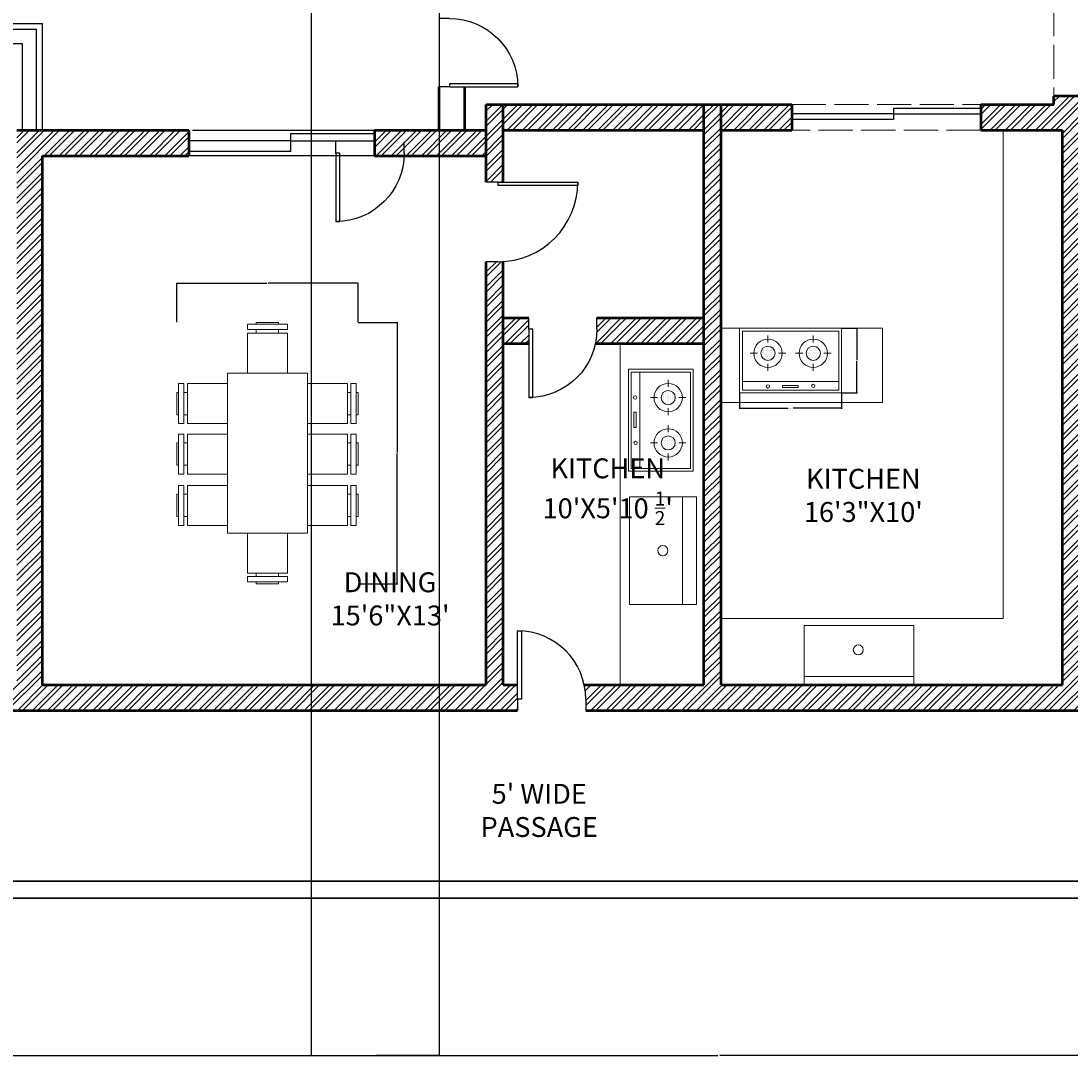
# Model space of a CAD drawing. Units: inches. Extents: x -249 to 953, y -127 to 590.
# Tile 2 of 4: x 171 to 540, y -127 to 237. Entities that reach past the tile are written whole.
import ezdxf

# ---------------------------------------------------------------- set-up
doc = ezdxf.new("R2010")
doc.units = ezdxf.units.IN
doc.header["$MEASUREMENT"] = 0
doc.linetypes.add('ACAD_ISO02W100', pattern=[15, 12, -3])
for name, color, linetype, lineweight in [('A-ANNO-DIMS', 2, 'Continuous', 18), ('A-AREA-IDEN', 2, 'Continuous', 18), ('A-EQPM', 249, 'Continuous', 18), ('A-FLOR-CASE', 8, 'Continuous', 18), ('A-FLOR-FIXT', 2, 'Continuous', 18), ('A-FURN', 42, 'Continuous', 18), ('A-GLAZ', 5, 'Continuous', 25), ('A-GLAZ-OVHD', 5, 'ACAD_ISO02W100', 18), ('A-WALL', 7, 'Continuous', 50), ('A-WALL-OVHD', 7, 'ACAD_ISO02W100', 18), ('A-WALL-PATT', 8, 'Continuous', 13), ('C-PROP', 7, 'Continuous', 35), ('DOOR', 22, 'Continuous', 25), ('L-ANNO-TEXT', 2, 'Continuous', 18)]:
    doc.layers.add(name, color=color, linetype=linetype, lineweight=lineweight)
doc.styles.get("Standard").update_dxf_attribs({"font": 'arial.ttf'})
doc.dimstyles.get("Standard").update_dxf_attribs({"dimtxt": 0.18, "dimasz": 0.18, "dimexe": 0.18, "dimexo": 0.0625, "dimgap": 0.09, "dimtad": 0, "dimtih": 1, "dimtoh": 1, "dimdec": 4, "dimzin": 0, "dimdsep": 46, "dimtxsty": 'Standard', "dimcen": 0.09, "dimadec": 0, "dimazin": 0, "dimtfac": 1, "dimtdec": 4, "dimtofl": 0, "dimtmove": 0, "dimatfit": 3, "dimfxl": 1, "dimtolj": 1, "dimtzin": 0, "dimarcsym": 0})

# ---------------------------------------------------------------- blocks, each defined once
blk = doc.blocks.new('*U2')
for p, q in [((0, 0), (0, -6)), ((40, 0), (40, -6))]:
    blk.add_line(p, q)
blk.add_lwpolyline([(0, 0), (0, 40), (1.75, 40), (1.75, 0)], close=True)
blk.add_arc((0, 0), 40, 0, 90)
blk = doc.blocks.new('A$C4C0603CD')
for p, q in [((1.106, 2.02), (0.656, 2.02)), ((0.656, 2.02), (0.656, 1.96)), ((1.006, 2.04), (0.756, 2.04)), ((0.756, 2.04), (0.756, 2.02)), ((1.006, 2.02), (1.006, 2.04)), ((1.106, 1.96), (1.106, 2.02)), ((1.232, 2.02), (1.232, 1.96)), ((1.684, 2.02), (1.232, 2.02)), ((1.584, 2.04), (1.334, 2.04)), ((1.334, 2.04), (1.334, 2.02)), ((1.584, 2.02), (1.584, 2.04)), ((1.684, 1.96), (1.684, 2.02)), ((1.802, 2.02), (1.802, 1.96)), ((2.252, 2.02), (1.802, 2.02)), ((2.152, 2.04), (1.902, 2.04)), ((1.902, 2.04), (1.902, 2.02)), ((2.152, 2.02), (2.152, 2.04)), ((2.252, 1.96), (2.252, 2.02)), ((1.106, 1.96), (0.656, 1.96)), ((0.656, 1.92), (0.656, 1.47)), ((1.106, 1.92), (0.656, 1.92)), ((0.756, 1.96), (0.756, 1.92)), ((1.006, 1.92), (1.006, 1.96)), ((1.106, 1.47), (1.106, 1.92)), ((1.684, 1.96), (1.232, 1.96)), ((1.232, 1.92), (1.232, 1.47)), ((1.684, 1.92), (1.232, 1.92)), ((1.334, 1.96), (1.334, 1.92)), ((1.584, 1.92), (1.584, 1.96)), ((1.684, 1.47), (1.684, 1.92)), ((2.252, 1.96), (1.802, 1.96)), ((1.802, 1.92), (1.802, 1.47)), ((2.252, 1.92), (1.802, 1.92)), ((1.902, 1.96), (1.902, 1.92)), ((2.152, 1.92), (2.152, 1.96)), ((2.252, 1.47), (2.252, 1.92)), ((0.57, 1.47), (0.57, 0.57)), ((2.37, 1.47), (0.57, 1.47)), ((0.656, 1.47), (1.106, 1.47)), ((1.107, 1.47), (1.684, 1.47)), ((1.802, 1.47), (2.252, 1.47)), ((2.37, 1.47), (2.37, 0.57)), ((0.02, 1.245), (0.02, 0.795)), ((0.08, 1.245), (0.02, 1.245)), ((0.08, 1.245), (0.08, 0.795)), ((0.12, 1.245), (0.12, 0.795)), ((0.57, 1.245), (0.12, 1.245)), ((0.57, 0.795), (0.57, 1.245)), ((2.37, 1.245), (2.37, 0.795)), ((2.82, 1.245), (2.37, 1.245)), ((2.82, 0.795), (2.82, 1.245)), ((2.86, 0.795), (2.86, 1.245)), ((2.92, 1.245), (2.86, 1.245)), ((2.92, 0.795), (2.92, 1.245)), ((0, 1.145), (0, 0.895)), ((0.02, 1.145), (0, 1.145)), ((0.12, 1.145), (0.08, 1.145)), ((2.86, 1.145), (2.82, 1.145)), ((2.94, 1.145), (2.92, 1.145)), ((2.94, 0.895), (2.94, 1.145)), ((0, 0.895), (0.02, 0.895)), ((0.08, 0.895), (0.12, 0.895)), ((2.82, 0.895), (2.86, 0.895)), ((2.92, 0.895), (2.94, 0.895)), ((0.02, 0.795), (0.08, 0.795)), ((0.12, 0.795), (0.57, 0.795)), ((2.37, 0.795), (2.82, 0.795)), ((2.86, 0.795), (2.92, 0.795)), ((0.57, 0.57), (2.37, 0.57)), ((1.106, 0.57), (0.656, 0.57)), ((0.656, 0.57), (0.656, 0.12)), ((1.106, 0.12), (1.106, 0.57)), ((1.684, 0.57), (1.232, 0.57)), ((1.232, 0.57), (1.232, 0.12)), ((1.684, 0.12), (1.684, 0.57)), ((2.252, 0.57), (1.802, 0.57)), ((1.802, 0.57), (1.802, 0.12)), ((2.252, 0.12), (2.252, 0.57)), ((0.656, 0.12), (1.106, 0.12)), ((0.756, 0.12), (0.756, 0.08)), ((1.006, 0.08), (1.006, 0.12)), ((1.232, 0.12), (1.684, 0.12)), ((1.334, 0.12), (1.334, 0.08)), ((1.584, 0.08), (1.584, 0.12)), ((1.802, 0.12), (2.252, 0.12)), ((1.902, 0.12), (1.902, 0.08)), ((2.152, 0.08), (2.152, 0.12)), ((0.656, 0.08), (1.106, 0.08)), ((0.656, 0.08), (0.656, 0.02)), ((0.656, 0.02), (1.106, 0.02)), ((0.756, 0.02), (0.756, 0)), ((0.756, 0), (1.006, 0)), ((1.006, 0), (1.006, 0.02)), ((1.106, 0.02), (1.106, 0.08)), ((1.232, 0.08), (1.684, 0.08)), ((1.232, 0.08), (1.232, 0.02)), ((1.232, 0.02), (1.684, 0.02)), ((1.334, 0.02), (1.334, 0)), ((1.334, 0), (1.584, 0)), ((1.584, 0), (1.584, 0.02)), ((1.684, 0.02), (1.684, 0.08)), ((1.802, 0.08), (2.252, 0.08)), ((1.802, 0.08), (1.802, 0.02)), ((1.802, 0.02), (2.252, 0.02)), ((1.902, 0.02), (1.902, 0)), ((1.902, 0), (2.152, 0)), ((2.152, 0), (2.152, 0.02)), ((2.252, 0.02), (2.252, 0.08))]:
    blk.add_line(p, q)
blk = doc.blocks.new('A$C475E21CF')
for p, q in [((0, 444.5), (0, 0)), ((0, 444.5), (699.9, 444.5)), ((699.9, 444.5), (699.9, 0)), ((19.4, 425), (19.4, 19.4)), ((19.4, 425), (680.5, 425)), ((194.5, 393.9), (194.5, 345.2)), ((505.4, 393.9), (505.4, 345.2)), ((680.5, 425), (680.5, 19.4)), ((160.9, 288.4), (160.9, 288.4)), ((166.9, 300.5), (166.9, 300.5)), ((173, 288.4), (173, 288.4)), ((179.1, 300.5), (179.1, 300.5)), ((185.2, 312.7), (185.2, 312.7)), ((185.2, 288.4), (185.2, 288.4)), ((191.2, 300.5), (191.2, 300.5)), ((197.3, 312.7), (197.3, 312.7)), ((197.3, 288.4), (197.3, 288.4)), ((203.4, 300.5), (203.4, 300.5)), ((209.5, 312.7), (209.5, 312.7)), ((209.5, 288.4), (209.5, 288.4)), ((215.6, 300.5), (215.6, 300.5)), ((221.6, 288.4), (221.6, 288.4)), ((227.7, 300.5), (227.7, 300.5)), ((233.8, 288.4), (233.8, 288.4)), ((474.1, 292.3), (474.1, 292.3)), ((480.2, 304.5), (480.2, 304.5)), ((486.3, 292.3), (486.3, 292.3)), ((492.3, 304.5), (492.3, 304.5)), ((498.4, 316.6), (498.4, 316.6)), ((498.4, 292.3), (498.4, 292.3)), ((504.5, 304.5), (504.5, 304.5)), ((510.6, 316.6), (510.6, 316.6)), ((510.6, 292.3), (510.6, 292.3)), ((516.7, 304.5), (516.7, 304.5)), ((522.7, 316.6), (522.7, 316.6)), ((522.7, 292.3), (522.7, 292.3)), ((528.8, 304.5), (528.8, 304.5)), ((534.9, 292.3), (534.9, 292.3)), ((541, 304.5), (541, 304.5)), ((547, 292.3), (547, 292.3)), ((72.9, 272.3), (121.6, 272.3)), ((148.7, 264.1), (148.7, 264.1)), ((154.8, 276.2), (154.8, 276.2)), ((154.8, 251.9), (154.8, 251.9)), ((160.9, 264.1), (160.9, 264.1)), ((160.9, 239.8), (160.9, 239.8)), ((166.9, 276.2), (166.9, 276.2)), ((166.9, 251.9), (166.9, 251.9)), ((173, 264.1), (173, 264.1)), ((173, 239.8), (173, 239.8)), ((179.1, 276.2), (179.1, 276.2)), ((179.1, 251.9), (179.1, 251.9)), ((179.1, 227.6), (179.1, 227.6)), ((185.2, 264.1), (185.2, 264.1)), ((185.2, 239.8), (185.2, 239.8)), ((191.2, 276.2), (191.2, 276.2)), ((191.2, 251.9), (191.2, 251.9)), ((191.2, 227.6), (191.2, 227.6)), ((197.3, 264.1), (197.3, 264.1)), ((197.3, 239.8), (197.3, 239.8)), ((203.4, 276.2), (203.4, 276.2)), ((203.4, 251.9), (203.4, 251.9)), ((203.4, 227.6), (203.4, 227.6)), ((209.5, 264.1), (209.5, 264.1)), ((209.5, 239.8), (209.5, 239.8)), ((215.6, 276.2), (215.6, 276.2)), ((215.6, 251.9), (215.6, 251.9)), ((215.6, 227.6), (215.6, 227.6)), ((221.6, 264.1), (221.6, 264.1)), ((221.6, 239.8), (221.6, 239.8)), ((227.7, 276.2), (227.7, 276.2)), ((227.7, 251.9), (227.7, 251.9)), ((233.8, 264.1), (233.8, 264.1)), ((233.8, 239.8), (233.8, 239.8)), ((239.9, 276.2), (239.9, 276.2)), ((239.9, 251.9), (239.9, 251.9)), ((267.4, 272.3), (316, 272.3)), ((383.9, 272.3), (432.5, 272.3)), ((462, 268), (462, 268)), ((468, 280.2), (468, 280.2)), ((468, 255.9), (468, 255.9)), ((474.1, 268), (474.1, 268)), ((474.1, 243.7), (474.1, 243.7)), ((480.2, 280.2), (480.2, 280.2)), ((480.2, 255.9), (480.2, 255.9)), ((486.3, 268), (486.3, 268)), ((486.3, 243.7), (486.3, 243.7)), ((492.3, 280.2), (492.3, 280.2)), ((492.3, 255.9), (492.3, 255.9)), ((492.3, 231.5), (492.3, 231.5)), ((498.4, 268), (498.4, 268)), ((498.4, 243.7), (498.4, 243.7)), ((504.5, 280.2), (504.5, 280.2)), ((504.5, 255.9), (504.5, 255.9)), ((504.5, 231.5), (504.5, 231.5)), ((510.6, 268), (510.6, 268)), ((510.6, 243.7), (510.6, 243.7)), ((516.7, 280.2), (516.7, 280.2)), ((516.7, 255.9), (516.7, 255.9)), ((516.7, 231.5), (516.7, 231.5)), ((522.7, 268), (522.7, 268)), ((522.7, 243.7), (522.7, 243.7)), ((528.8, 280.2), (528.8, 280.2)), ((528.8, 255.9), (528.8, 255.9)), ((528.8, 231.5), (528.8, 231.5)), ((534.9, 268), (534.9, 268)), ((534.9, 243.7), (534.9, 243.7)), ((541, 280.2), (541, 280.2)), ((541, 255.9), (541, 255.9)), ((547, 268), (547, 268)), ((547, 243.7), (547, 243.7)), ((553.1, 280.2), (553.1, 280.2)), ((553.1, 255.9), (553.1, 255.9)), ((578.4, 272.3), (627, 272.3)), ((194.5, 199.4), (194.5, 150.8)), ((505.4, 199.4), (505.4, 150.8)), ((19.4, 77.8), (680.5, 77.8)), ((0, 0), (699.9, 0)), ((19.4, 19.4), (680.5, 19.4)), ((293.4, 51.9), (400.6, 51.9)), ((293.4, 36.5), (293.4, 51.9)), ((400.6, 36.5), (293.4, 36.5)), ((400.6, 51.9), (400.6, 36.5))]:
    blk.add_line(p, q)
for centre, radius in [((194.5, 272.3), 97.2), ((505.4, 272.3), 97.2), ((194.5, 272.3), 48.6), ((505.4, 272.3), 48.6), ((193.9, 45.1), 11.7), ((505.2, 48.5), 11.7)]:
    blk.add_circle(centre, radius)
blk = doc.blocks.new('*U9')
for p, q in [((0, 0), (0, -5)), ((30, 0), (30, -5))]:
    blk.add_line(p, q)
blk.add_lwpolyline([(0, 0), (0, 30), (1.75, 30), (1.75, 0)], close=True)
blk.add_arc((0, 0), 30, 0, 90)
blk = doc.blocks.new('*D35')
at = {"layer": 'A-ANNO-DIMS', "color": 0, "lineweight": -2, "transparency": 16777216}
for p, q in [((423.75, 106.47), (423.75, 100.98)), ((459.62, 106.47), (459.62, 100.98)), ((423.93, 101.16), (440.86, 101.16)), ((459.44, 101.16), (442.52, 101.16))]:
    blk.add_line(p, q, dxfattribs=at)
at = {"layer": 'A-ANNO-DIMS', "color": 0, "transparency": 16777216}
for points in [[(423.93, 101.19), (423.93, 101.13), (423.75, 101.16)], [(459.44, 101.19), (459.44, 101.13), (459.62, 101.16)]]:
    blk.add_solid(points, dxfattribs=at)
at = {"layer": 'Defpoints', "color": 0, "transparency": 16777216}
for p in [(423.75, 106.54), (459.62, 106.54), (459.62, 101.16)]:
    blk.add_point(p, dxfattribs=at)
at = {"layer": 'A-ANNO-DIMS', "color": 0, "transparency": 16777216, "insert": (441.69, 101.16), "char_height": 0.18, "attachment_point": 5}
blk.add_mtext('\\A1;HOB 36 TYP.', dxfattribs=at)
blk = doc.blocks.new('*D36')
at = {"layer": 'A-ANNO-DIMS', "color": 0, "lineweight": -2, "transparency": 16777216}
for p, q in [((459.68, 129.31), (465.18, 129.31)), ((465, 129.13), (465, 118.11)), ((465, 106.72), (465, 117.74)), ((459.68, 106.54), (465.18, 106.54))]:
    blk.add_line(p, q, dxfattribs=at)
at = {"layer": 'A-ANNO-DIMS', "color": 0, "transparency": 16777216}
for points in [[(464.97, 129.13), (465.03, 129.13), (465, 129.31)], [(464.97, 106.72), (465.03, 106.72), (465, 106.54)]]:
    blk.add_solid(points, dxfattribs=at)
at = {"layer": 'Defpoints', "color": 0, "transparency": 16777216}
for p in [(459.62, 129.31), (465, 129.31), (459.62, 106.54)]:
    blk.add_point(p, dxfattribs=at)
at = {"layer": 'A-ANNO-DIMS', "color": 0, "transparency": 16777216, "insert": (465, 117.93), "char_height": 0.18, "attachment_point": 5}
blk.add_mtext('\\A1;23 TYP.', dxfattribs=at)
blk = doc.blocks.new('*D45')
at = {"layer": 'A-ANNO-DIMS', "color": 0, "lineweight": -2, "transparency": 16777216}
for p, q in [((289.73, 131.32), (303.63, 131.32)), ((303.45, 131.14), (303.45, 85.59)), ((303.45, 39.67), (303.45, 85.22)), ((289.73, 39.49), (303.63, 39.49))]:
    blk.add_line(p, q, dxfattribs=at)
at = {"layer": 'A-ANNO-DIMS', "color": 0, "transparency": 16777216}
for points in [[(303.42, 131.14), (303.48, 131.14), (303.45, 131.32)], [(303.42, 39.67), (303.48, 39.67), (303.45, 39.49)]]:
    blk.add_solid(points, dxfattribs=at)
at = {"layer": 'Defpoints', "color": 0, "transparency": 16777216}
for p in [(289.67, 131.32), (303.45, 131.32), (289.67, 39.49)]:
    blk.add_point(p, dxfattribs=at)
at = {"layer": 'A-ANNO-DIMS', "color": 0, "transparency": 16777216, "insert": (303.45, 85.4), "char_height": 0.18, "attachment_point": 5}
blk.add_mtext('\\A1;DINING SET 92', dxfattribs=at)
blk = doc.blocks.new('*D46')
at = {"layer": 'A-ANNO-DIMS', "color": 0, "lineweight": -2, "transparency": 16777216}
for p, q in [((225.95, 131.38), (225.95, 145.27)), ((226.13, 145.09), (257.59, 145.09)), ((289.49, 145.09), (258.03, 145.09)), ((289.67, 131.38), (289.67, 145.27))]:
    blk.add_line(p, q, dxfattribs=at)
at = {"layer": 'A-ANNO-DIMS', "color": 0, "transparency": 16777216}
for points in [[(226.13, 145.12), (226.13, 145.06), (225.95, 145.09)], [(289.49, 145.12), (289.49, 145.06), (289.67, 145.09)]]:
    blk.add_solid(points, dxfattribs=at)
at = {"layer": 'Defpoints', "color": 0, "transparency": 16777216}
for p in [(225.95, 145.09), (225.95, 131.32), (289.67, 131.32)]:
    blk.add_point(p, dxfattribs=at)
at = {"layer": 'A-ANNO-DIMS', "color": 0, "transparency": 16777216, "insert": (257.81, 145.09), "char_height": 0.18, "attachment_point": 5}
blk.add_mtext('\\A1;64', dxfattribs=at)
blk = doc.blocks.new('*D53')
at = {"layer": 'A-ANNO-DIMS', "color": 0, "lineweight": -2, "transparency": 16777216}
for p, q in [((1.72, -5.13), (1.72, -126.55)), ((831.22, -5.13), (831.22, -126.55)), ((1.9, -126.37), (416.07, -126.37)), ((831.04, -126.37), (416.86, -126.37))]:
    blk.add_line(p, q, dxfattribs=at)
at = {"layer": 'A-ANNO-DIMS', "color": 0, "transparency": 16777216}
for points in [[(1.9, -126.34), (1.9, -126.4), (1.72, -126.37)], [(831.04, -126.34), (831.04, -126.4), (831.22, -126.37)]]:
    blk.add_solid(points, dxfattribs=at)
at = {"layer": 'Defpoints', "color": 0, "transparency": 16777216}
for p in [(1.72, -5.07), (831.22, -5.07), (831.22, -126.37)]:
    blk.add_point(p, dxfattribs=at)
at = {"layer": 'A-ANNO-DIMS', "color": 0, "transparency": 16777216, "insert": (416.47, -126.37), "char_height": 0.18, "attachment_point": 5}
blk.add_mtext('\\A1;829.5', dxfattribs=at)
blk = doc.blocks.new('*D59')
at = {"layer": 'A-ANNO-DIMS', "color": 0, "lineweight": -2, "transparency": 16777216}
for p, q in [((273.22, 325.87), (273.22, -126.55)), ((318.22, 325.87), (318.22, -126.55)), ((273.4, -126.37), (295.49, -126.37)), ((318.04, -126.37), (295.94, -126.37))]:
    blk.add_line(p, q, dxfattribs=at)
at = {"layer": 'A-ANNO-DIMS', "color": 0, "transparency": 16777216}
for points in [[(273.4, -126.34), (273.4, -126.4), (273.22, -126.37)], [(318.04, -126.34), (318.04, -126.4), (318.22, -126.37)]]:
    blk.add_solid(points, dxfattribs=at)
at = {"layer": 'Defpoints', "color": 0, "transparency": 16777216}
for p in [(273.22, 325.93), (318.22, 325.93), (318.22, -126.37)]:
    blk.add_point(p, dxfattribs=at)
at = {"layer": 'A-ANNO-DIMS', "color": 0, "transparency": 16777216, "insert": (295.72, -126.37), "char_height": 0.18, "attachment_point": 5}
blk.add_mtext('\\A1;45', dxfattribs=at)

msp = doc.modelspace()

# ---------------------------------------------------------------- hatches: boundary and pattern name
at = {"layer": 'A-WALL-PATT'}
h = msp.add_hatch(dxfattribs=at)
h.set_pattern_fill('ANSI32', color=256, scale=10)
h.paths.add_polyline_path([(765.2157, 3.9306), (708.2157, 3.9306), (708.2157, 114.9306), (699.2157, 114.9306), (699.2157, 3.9306), (546.2157, 3.9306), (546.2157, 54.9306), (576.2157, 54.9306), (576.2157, 63.9306), (546.2157, 63.9306), (546.2157, 105.9306), (576.2157, 105.9306), (576.2157, 114.9306), (543.2157, 114.9306), (543.2157, 210.9306), (534.2157, 210.9306), (534.2157, 207.9306), (508.5171, 207.9306), (508.5171, 198.9306), (537.2157, 198.9306), (537.2157, 3.9306), (417.2157, 3.9306), (417.2157, 207.9306), (411.2157, 207.9306), (411.2157, 3.9306), (369.1469, 3.9306, -0.05252224), (369.6736, -1.0697), (369.6736, -5.0694), (765.2157, -5.0694)])
h = msp.add_hatch(dxfattribs=at)
h.set_pattern_fill('ANSI32', color=256, scale=10)
h.paths.add_polyline_path([(442.0897, 207.9306), (417.2157, 207.9306), (417.2157, 198.9306), (442.0897, 198.9306)])
h.paths.add_polyline_path([(411.2157, 207.9306), (340.7157, 207.9306), (340.7157, 198.9306), (411.2157, 198.9306)])
h.paths.add_polyline_path([(340.7157, 207.9306), (334.7157, 207.9306), (334.7157, 180.6902), (338.9157, 180.6902), (340.7157, 180.6902)])
h.paths.add_polyline_path([(334.7157, 198.9306), (295.4153, 198.9306), (295.4153, 189.9306), (334.7157, 189.9306)], flags=17)
h.paths.add_polyline_path([(411.2157, 132.9306), (373.6294, 132.9306), (373.6294, 128.9308, -0.05252224), (373.1027, 123.9306), (411.2157, 123.9306)])
h.paths.add_polyline_path([(340.7157, 152.7481, -0.01608391), (338.9157, 152.6902), (334.7157, 152.6902), (334.7157, 3.9306), (178.7157, 3.9306), (178.7157, 189.9306), (230.1981, 189.9306), (230.1981, 198.9306), (169.7157, 198.9306), (169.7157, 3.9306), (10.7157, 3.9306), (10.7157, 62.26), (1.7157, 62.26), (1.7157, -5.0694), (345.6752, -5.0694), (345.6752, -1.0697), (345.6752, 3.9306), (340.7157, 3.9306)])
h.paths.add_polyline_path([(349.631, 132.9306), (340.7157, 132.9306), (340.7157, 123.9306), (349.631, 123.9306), (349.631, 128.9308)])

# ---------------------------------------------------------------- linework, layer by layer
at = {"layer": 'A-FLOR-CASE'}
for p, q in [((516.403, 198.9306), (516.403, 27.2666)), ((417.2157, 129.314), (417.2157, 129.314)), ((417.2157, 129.314), (473.9251, 129.314)), ((473.9251, 129.314), (473.9251, 103.1985)), ((381.7752, 123.9306), (381.7752, 3.9306)), ((473.9251, 103.1985), (417.2157, 103.1985)), ((516.403, 27.2666), (417.2157, 27.2666))]:
    msp.add_line(p, q, dxfattribs=at)
at = {"layer": 'A-FLOR-FIXT'}
for p, q in [((403.7051, 70.0228), (403.7051, 32.1897)), ((484.9386, 6.8463), (446.4336, 6.8463))]:
    msp.add_line(p, q, dxfattribs=at)
for points in [[(385.0212, 70.0228), (408.568, 70.0228), (408.568, 32.1897), (385.0212, 32.1897)], [(446.4336, 24.8323), (484.9386, 24.8323), (484.9386, 3.9306), (446.4336, 3.9306)]]:
    msp.add_lwpolyline(points, close=True, dxfattribs=at)
for centre, radius in [((396.7946, 51.1063), 1.7916), ((465.4665, 16.2049), 1.7569)]:
    msp.add_circle(centre, radius, dxfattribs=at)
at = {"layer": 'A-GLAZ'}
for p, q in [((162.2157, 236.4306), (178.7157, 236.4306)), ((178.7157, 198.9306), (178.7157, 236.4306)), ((162.2157, 234.4306), (176.7157, 234.4306)), ((176.7157, 198.9306), (176.7157, 234.4306)), ((162.2157, 229.4306), (171.7157, 229.4306)), ((171.7157, 198.9306), (171.7157, 229.4306)), ((477.8425, 204.617), (442.0897, 204.617)), ((508.5171, 206.5658), (477.8425, 206.5658)), ((477.8425, 206.5658), (477.8425, 202.6683)), ((477.8425, 204.617), (508.5171, 204.617)), ((477.8425, 202.6683), (442.0897, 202.6683)), ((231.5291, 198.9306), (295.4153, 198.9306)), ((265.964, 197.6756), (265.964, 191.4056)), ((295.4153, 197.6756), (265.964, 197.6756)), ((265.964, 195.1681), (230.1981, 195.1681)), ((265.964, 195.1681), (295.4153, 195.1681)), ((265.964, 191.4056), (230.1981, 191.4056)), ((295.4153, 189.9306), (230.1981, 189.9306))]:
    msp.add_line(p, q, dxfattribs=at)
at = {"layer": 'A-GLAZ-OVHD'}
for p, q in [((442.0897, 207.9306), (508.5171, 207.9306)), ((508.5171, 198.9306), (442.0897, 198.9306))]:
    msp.add_line(p, q, dxfattribs=at)
at = {"layer": 'A-WALL'}
for p, q in [((318.2157, 198.9306), (318.2157, 214.174)), ((327.2157, 198.9306), (327.2157, 214.174)), ((534.2157, 207.9306), (534.2157, 210.9306)), ((543.2157, 210.9306), (534.2157, 210.9306)), ((334.7157, 207.9306), (442.0897, 207.9306)), ((334.7157, 180.6902), (334.7157, 207.9306)), ((340.7157, 180.6902), (340.7157, 207.9306)), ((411.2157, 3.9306), (411.2157, 207.9306)), ((417.2157, 3.9306), (417.2157, 207.9306)), ((442.0897, 207.9306), (442.0897, 198.9306)), ((508.5171, 207.9306), (508.5171, 198.9306)), ((508.5171, 207.9306), (534.2157, 207.9306)), ((169.7157, 198.9306), (230.1981, 198.9306)), ((230.1981, 198.9306), (230.1981, 189.9306)), ((295.4153, 198.9306), (295.4153, 189.9306)), ((295.4153, 198.9306), (334.7157, 198.9306)), ((340.7157, 198.9306), (411.2157, 198.9306)), ((417.2157, 198.9306), (442.0897, 198.9306)), ((508.5171, 198.9306), (537.2157, 198.9306)), ((537.2157, 3.9306), (537.2157, 198.9306)), ((178.7157, 3.9306), (178.7157, 189.9306)), ((178.7157, 189.9306), (230.1981, 189.9306)), ((295.4153, 189.9306), (334.7157, 189.9306)), ((334.7157, 3.9306), (334.7157, 152.6902)), ((340.7157, 3.9306), (340.7157, 152.7481)), ((340.7157, 132.9306), (349.631, 132.9306)), ((373.6294, 132.9306), (411.2157, 132.9306)), ((340.7157, 123.9306), (349.631, 123.9306)), ((373.1027, 123.9306), (411.2157, 123.9306)), ((178.7157, 3.9306), (334.7157, 3.9306)), ((340.7157, 3.9306), (345.6752, 3.9306)), ((369.1469, 3.9306), (411.2157, 3.9306)), ((417.2157, 3.9306), (537.2157, 3.9306)), ((1.7157, -5.0694), (345.6752, -5.0694)), ((369.6736, -5.0694), (765.2157, -5.0694))]:
    msp.add_line(p, q, dxfattribs=at)
at = {"layer": 'A-WALL-OVHD'}
msp.add_line((534.2157, 258.9306), (534.2157, 210.9306), dxfattribs=at)
at = {"layer": 'C-PROP'}
for p, q in [((-187.2843, -65.0694), (891.2157, -65.0694)), ((-193.2843, -71.0694), (897.2157, -71.0694))]:
    msp.add_line(p, q, dxfattribs=at)

# ---------------------------------------------------------------- block references
at = {"layer": 'A-EQPM', "xscale": 0.0512434632309567, "yscale": 0.0512434632309567, "zscale": 0.0512434632309567}
msp.add_blockref('A$C475E21CF', (423.7546, 106.5366), dxfattribs=at)
at = {"layer": 'A-EQPM', "xscale": 0.0512434632309567, "yscale": 0.0512434632309567, "zscale": 0.0512434632309567, "rotation": 270}
msp.add_blockref('A$C475E21CF', (384.7055, 114.8797), dxfattribs=at)
at = {"layer": 'A-FURN', "xscale": 31.23529604178421, "yscale": 31.23529604178421, "zscale": 31.23529604178421, "rotation": 90}
msp.add_blockref('A$C4C0603CD', (289.6704, 39.4875), dxfattribs=at)
at = {"layer": 'DOOR'}
for name, p, xscale, yscale, zscale, rotation in [('*U2', (321.8157, 214.174), -0.6, 0.6, 0.6, 270), ('*U9', (281.863, 190.7883), -0.7999467951057515, 0.7999467951057515, 0.7999467951057515, 180), ('*U2', (338.9157, 180.6902), 0.7000000000000001, 0.7000000000000001, 0.7000000000000001, 270), ('*U9', (349.631, 128.9308), -0.7999467951057515, 0.7999467951057515, 0.7999467951057515, 180)]:
    msp.add_blockref(name, p, dxfattribs=dict(at, xscale=xscale, yscale=yscale, zscale=zscale, rotation=rotation))
at = {"layer": 'DOOR', "xscale": 0.7999467951057515, "yscale": 0.7999467951057515, "zscale": 0.7999467951057515}
msp.add_blockref('*U9', (345.6752, -1.0697), dxfattribs=at)

# ---------------------------------------------------------------- texts
at = {"layer": 'A-AREA-IDEN', "char_height": 7, "attachment_point": 1}
for s, insert in [("\\A1;\\pxqc;KITCHEN\\P10'X5'10 {\\H0.7x;\\S1/2;}'", (337.6058, 83.5378)), ('\\A1;\\pxqc;KITCHEN\\P16\'3"X10\'', (427.4325, 79.874)), ('\\A1;\\pxqc;DINING\\P15\'6"X13\'', (261.1058, 43.4904))]:
    msp.add_mtext_dynamic_manual_height_columns(s, width=79.609867, gutter_width=1, heights=[0], dxfattribs=dict(at, insert=insert))
at = {"layer": 'L-ANNO-TEXT', "insert": (313.5386, -30.8785), "char_height": 7, "attachment_point": 1}
msp.add_mtext_dynamic_manual_height_columns("\\A1;\\pxqc;5' WIDE\\PPASSAGE", width=79.609867, gutter_width=1, heights=[0], dxfattribs=at)

# ---------------------------------------------------------------- dimensions: what is measured, and where the dimension line sits
at = {"layer": 'A-ANNO-DIMS'}
for base, p1, p2, override, picture, middle in [((318.2157, -126.3694), (273.2157, 325.9306), (318.2157, 325.9306), {"dimdec": 0, "dimlfac": 1, "dimrnd": 0, "dimzin": 0, "dimdsep": 46, "dimlunit": 2}, '*D59', (295.7157, -126.3694)), ((831.2157, -126.3694), (1.7157, -5.0694), (831.2157, -5.0694), {"dimdec": 1, "dimlfac": 1, "dimrnd": 0, "dimzin": 0, "dimdsep": 46, "dimlunit": 2}, '*D53', (416.4657, -126.3694))]:
    dim = msp.add_linear_dim(base=base, p1=p1, p2=p2, dimstyle='Standard', override=override, dxfattribs=at)
    dim.commit()
    dim.dimension.update_dxf_attribs({"geometry": picture, "text_midpoint": middle})
dim = msp.add_linear_dim(base=(225.9504, 145.0941), p1=(289.6704, 131.3193), p2=(225.9504, 131.3193), angle=180, dimstyle='Standard', override={"dimdec": 0, "dimlfac": 1, "dimrnd": 0, "dimzin": 0, "dimdsep": 46, "dimlunit": 2}, dxfattribs=at)
dim.commit()
dim.dimension.update_dxf_attribs({"geometry": '*D46', "text_midpoint": (257.8104, 145.0941)})
for base, p1, p2, text, picture, middle in [((303.4452, 131.3193), (289.6704, 39.4875), (289.6704, 131.3193), 'DINING SET <>', '*D45', (303.4452, 85.4034)), ((465.0011, 129.314), (459.6211, 106.5366), (459.6211, 129.314), '<> TYP.', '*D36', (465.0011, 117.9253))]:
    dim = msp.add_linear_dim(base=base, p1=p1, p2=p2, angle=90, text=text, dimstyle='Standard', override={"dimdec": 0, "dimlfac": 1, "dimrnd": 0, "dimzin": 0, "dimdsep": 46, "dimlunit": 2}, dxfattribs=at)
    dim.commit()
    dim.dimension.update_dxf_attribs({"geometry": picture, "text_midpoint": middle})
dim = msp.add_linear_dim(base=(459.6211, 101.1567), p1=(423.7546, 106.5366), p2=(459.6211, 106.5366), text='HOB <> TYP.', dimstyle='Standard', override={"dimdec": 0, "dimlfac": 1, "dimrnd": 0, "dimzin": 0, "dimdsep": 46, "dimlunit": 2}, dxfattribs=at)
dim.commit()
dim.dimension.update_dxf_attribs({"geometry": '*D35', "text_midpoint": (441.6878, 101.1567)})

doc.saveas('drawing.dxf')
